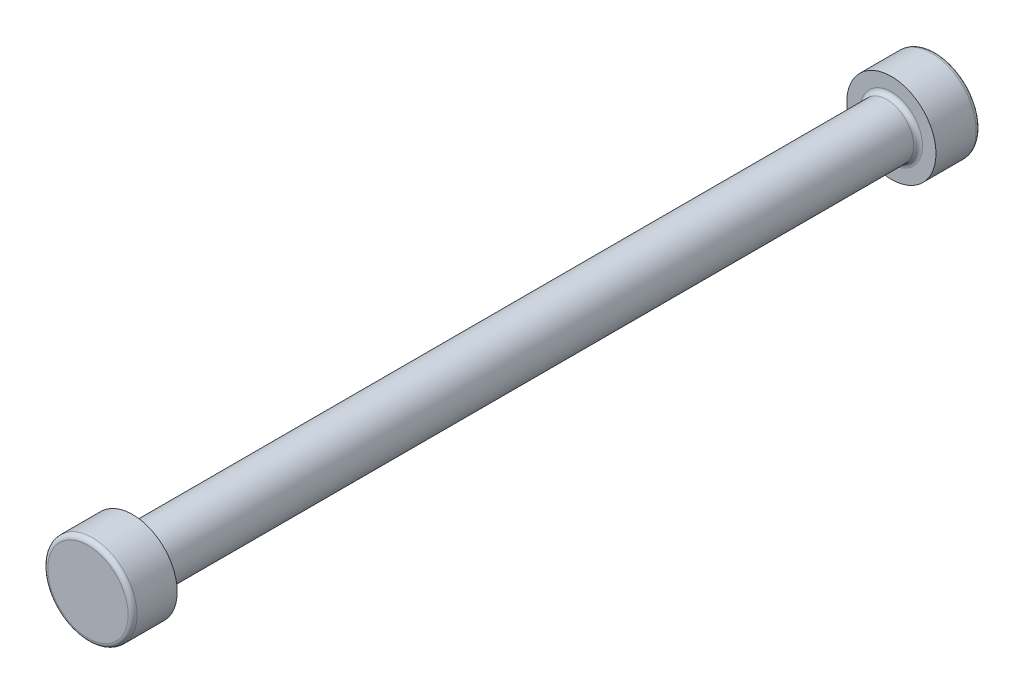
from build123d import *

# Parameters (mm, degrees)
SHAFT_PROFILE_6_R        = 3
SHAFT_6X95_DEPTH         = 47.5
HEAD_PROFILE_10_R        = 5
HEAD_10X5_DEPTH          = 5
HEAD_EDGE_FILLETS_R0_5_R = 0.5


with BuildPart() as part:
    # Shaft Profile Ø6 → Shaft Ø6x95 (new, symmetric)
    with BuildSketch(Plane.XY):
        Circle(SHAFT_PROFILE_6_R)
    extrude(amount=SHAFT_6X95_DEPTH, both=True)

    # Head Profile Ø10 → Head Ø10x5 (add)
    with BuildSketch(Plane.XY.offset(47.5)):
        Circle(HEAD_PROFILE_10_R)
    head_10x5 = extrude(amount=-HEAD_10X5_DEPTH)

    # Head Mirror: Head Ø10x5 across plane
    add(head_10x5.mirror(Plane.XY))

    # Head Edge Fillets R0.5
    head_edge_fillets_r0_5_edges = [part.edges().sort_by_distance(p)[0] for p in [
        (-3, 0, -42.5),
        (-5, 0, -47.5),
        (-3, 0, 42.5),
        (-5, 0, 47.5),
    ]]
    fillet(head_edge_fillets_r0_5_edges, radius=HEAD_EDGE_FILLETS_R0_5_R)


solid = part.part
